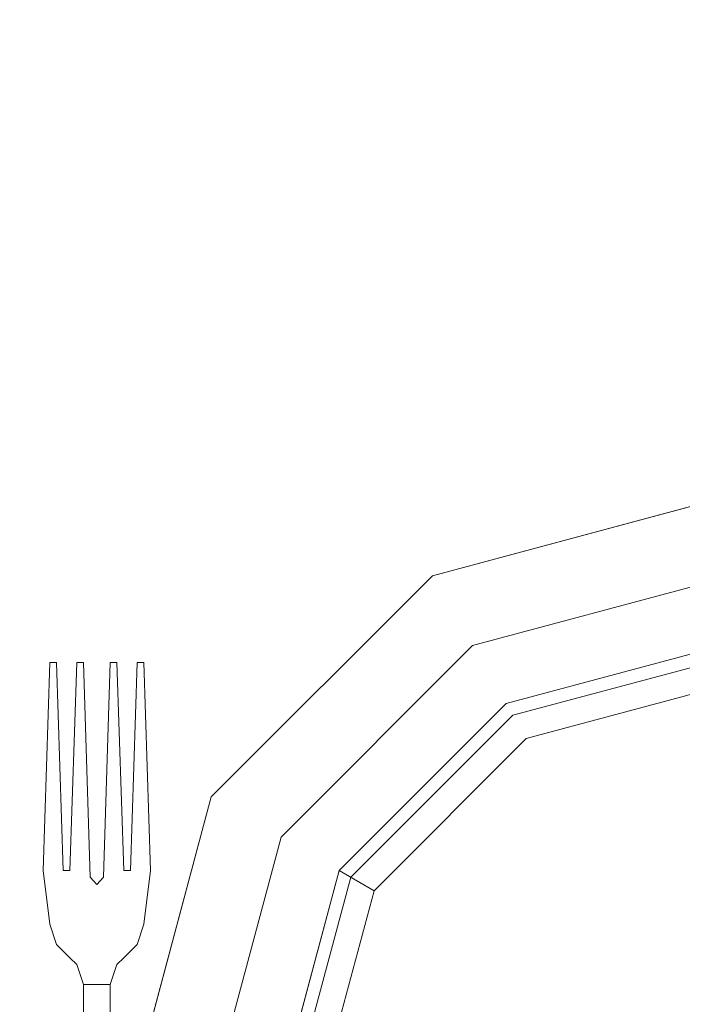
# Model space of a CAD drawing. Units: inches. Extents: x 375 to 1122, y 27 to 1069.
# Tile 87 of 155: x 719.125 to 725.203, y 854.634 to 863.668. Entities that reach past the tile are written whole.
import ezdxf

# ---------------------------------------------------------------- set-up
doc = ezdxf.new("R2010")
doc.units = ezdxf.units.IN
doc.layers.add('A-ANNO-DIMS', color=2, linetype='Continuous', lineweight=18)
doc.layers.add('Furniture', color=30, linetype='Continuous', lineweight=18)
doc.styles.get("Standard").update_dxf_attribs({"font": 'arial.ttf'})
doc.dimstyles.new('ISO-25', dxfattribs={"dimtxt": 12, "dimasz": 2.5, "dimexe": 1.5, "dimexo": 1.5, "dimtad": 1, "dimdec": 1, "dimlunit": 3, "dimtxsty": 'Standard', "dimblk": 'ARCHTICK', "dimcen": 2.5, "dimadec": 0, "dimazin": 0, "dimtfac": 1, "dimtdec": 1, "dimtmove": 0, "dimatfit": 3, "dimfxl": 1.5, "dimfxlon": 1, "dimarcsym": 0})

# ---------------------------------------------------------------- blocks, each defined once
blk = doc.blocks.new('A$C403C54AD')
for p, q in [((2.0741, 0.86135, -0.05014), (2.07871, 0.86289, -0.04968)), ((2.0741, 0.86135, -0.05322), (2.07871, 0.86289, -0.05276))]:
    blk.add_line(p, q)
at = {"linetype": 'ByBlock'}
for points, invisible_edges in [([(1.97559, 1.01834, -0.03783), (1.99406, 1.01834, -0.03783), (2.01014, 0.95832, -0.03783), (1.99415, 0.94908, -0.03783)], 5), ([(2.00945, 1.01834, -0.05168), (1.97559, 1.01834, -0.04244), (1.99415, 0.94908, -0.04244), (2.02347, 0.96601, -0.05168)], 5), ([(1.99406, 1.01834, -0.03783), (2.01253, 1.01834, -0.04398), (2.02614, 0.96755, -0.04398), (2.01014, 0.95832, -0.03783)], 5), ([(2.01868, 1.01834, -0.06091), (2.00945, 1.01834, -0.05168), (2.02347, 0.96601, -0.05168), (2.03147, 0.97063, -0.06091)], 5), ([(2.01253, 1.01834, -0.04398), (2.11411, 1.01834, -0.04398), (2.11411, 1.01834, -0.04398), (2.02614, 0.96755, -0.04398)], 5), ([(2.02614, 0.96755, -0.04398), (2.11411, 1.01834, -0.04398), (2.11411, 1.01834, -0.04398), (2.06332, 0.93037, -0.04398)], 5), ([(2.06332, 0.93037, -0.04398), (2.11411, 1.01834, -0.04398), (2.11411, 1.01834, -0.04398), (2.11411, 0.91676, -0.04398)], 5), ([(2.03147, 0.97063, -0.06091), (2.02347, 0.96601, -0.05168), (2.06178, 0.9277, -0.05168), (2.0664, 0.9357, -0.06091)], 1), ([(2.01014, 0.95832, -0.03783), (2.02614, 0.96755, -0.04398), (2.06332, 0.93037, -0.04398), (2.05409, 0.91437, -0.03783)], 5), ([(2.02347, 0.96601, -0.05168), (1.99415, 0.94908, -0.04244), (2.04485, 0.89838, -0.04244), (2.06178, 0.9277, -0.05168)], 5), ([(1.99415, 0.94908, -0.03783), (2.01014, 0.95832, -0.03783), (2.05409, 0.91437, -0.03783), (2.04485, 0.89838, -0.03783)], 5), ([(2.05409, 0.91437, -0.03783), (2.06332, 0.93037, -0.04398), (2.11411, 0.91676, -0.04398), (2.11411, 0.89829, -0.03783)], 5), ([(2.06178, 0.9277, -0.05168), (2.04485, 0.89838, -0.04244), (2.11411, 0.87982, -0.04244), (2.11411, 0.91368, -0.05168)], 5), ([(2.04485, 0.89838, -0.03783), (2.05409, 0.91437, -0.03783), (2.11411, 0.89829, -0.03783), (2.11411, 0.87982, -0.03783)], 5)]:
    blk.add_3dface(points, dxfattribs=dict(at, invisible_edges=invisible_edges))
for points in [[(1.97559, 1.01834, -0.04244), (1.97559, 1.01834, -0.03783), (1.99415, 0.94908, -0.03783), (1.99415, 0.94908, -0.04244)], [(1.99415, 0.94908, -0.04244), (1.99415, 0.94908, -0.03783), (2.04485, 0.89838, -0.03783), (2.04485, 0.89838, -0.04244)], [(2.0664, 0.9357, -0.06091), (2.06178, 0.9277, -0.05168), (2.11411, 0.91368, -0.05168), (2.11411, 0.92291, -0.06091)], [(2.04485, 0.89838, -0.04244), (2.04485, 0.89838, -0.03783), (2.11411, 0.87982, -0.03783), (2.11411, 0.87982, -0.04244)]]:
    blk.add_3dface(points, dxfattribs=at)
for points, invisible_edges in [([(2.06178, 0.87982, -0.04954), (2.06178, 0.88444, -0.04954), (2.01407, 0.8829, -0.04244), (2.01407, 0.88136, -0.04244)], 1), ([(2.06178, 0.87982, -0.05262), (2.06178, 0.88444, -0.05262), (2.01407, 0.8829, -0.04552), (2.01407, 0.88136, -0.04552)], 1), ([(2.0741, 0.8829, -0.05014), (2.06178, 0.87828, -0.04954), (2.06178, 0.87982, -0.04954), (2.06178, 0.88444, -0.04954)], 5), ([(2.0741, 0.8829, -0.05322), (2.06178, 0.87828, -0.05262), (2.06178, 0.87982, -0.05262), (2.06178, 0.88444, -0.05262)], 5), ([(2.0741, 0.8829, -0.05014), (2.0741, 0.8829, -0.05322), (2.06178, 0.88444, -0.05262), (2.06178, 0.88444, -0.04954)], 1), ([(2.0741, 0.8829, -0.05014), (2.06498, 0.87212, -0.04994), (2.06332, 0.87366, -0.04979), (2.06178, 0.87828, -0.04954)], 13), ([(2.0741, 0.8829, -0.05322), (2.06498, 0.87212, -0.05301), (2.06332, 0.87366, -0.05286), (2.06178, 0.87828, -0.05262)], 13), ([(2.0741, 0.8829, -0.05014), (2.06498, 0.87212, -0.04994), (2.0741, 0.86135, -0.05014), (2.0741, 0.8829, -0.05014)], 7), ([(2.0741, 0.8829, -0.05322), (2.06498, 0.87212, -0.05301), (2.0741, 0.86135, -0.05322), (2.0741, 0.8829, -0.05322)], 7), ([(2.07871, 0.88136, -0.04968), (2.07871, 0.86289, -0.04968), (2.0741, 0.86135, -0.05014), (2.0741, 0.8829, -0.05014)], 5), ([(2.07871, 0.88136, -0.05276), (2.07871, 0.86289, -0.05276), (2.0741, 0.86135, -0.05322), (2.0741, 0.8829, -0.05322)], 5), ([(2.07871, 0.88136, -0.05276), (2.07871, 0.88136, -0.04968), (2.0741, 0.8829, -0.05014), (2.0741, 0.8829, -0.05322)], 4), ([(2.08179, 0.86596, -0.05152), (2.08179, 0.87828, -0.05152), (2.07871, 0.88136, -0.05276), (2.07871, 0.86289, -0.05276)], 5), ([(2.08179, 0.86596, -0.04844), (2.08179, 0.87828, -0.04844), (2.07871, 0.88136, -0.04968), (2.07871, 0.86289, -0.04968)], 5), ([(2.06178, 0.87828, -0.04954), (2.06332, 0.87366, -0.04979), (2.01407, 0.8752, -0.04244), (2.01407, 0.87674, -0.04244)], 1), ([(2.06178, 0.87828, -0.05262), (2.06332, 0.87366, -0.05286), (2.01407, 0.8752, -0.04552), (2.01407, 0.87674, -0.04552)], 1), ([(2.08333, 0.8675, -0.04739), (2.08333, 0.87674, -0.04739), (2.08179, 0.87828, -0.04844), (2.08179, 0.86596, -0.04844)], 5), ([(2.08333, 0.8675, -0.05018), (2.08333, 0.87674, -0.05018), (2.08179, 0.87828, -0.05152), (2.08179, 0.86596, -0.05152)], 5), ([(2.08333, 0.87674, -0.05018), (2.08333, 0.87674, -0.04739), (2.08179, 0.87828, -0.04844), (2.08179, 0.87828, -0.05152)], 1), ([(2.08795, 0.8752, -0.04504), (2.08795, 0.86904, -0.04504), (2.08333, 0.8675, -0.04739), (2.08333, 0.87674, -0.04739)], 4), ([(2.08795, 0.8752, -0.04504), (2.08795, 0.8752, -0.04763), (2.08333, 0.87674, -0.05018), (2.08333, 0.87674, -0.04739)], 5), ([(2.08795, 0.8752, -0.04763), (2.08795, 0.86904, -0.04763), (2.08333, 0.8675, -0.05018), (2.08333, 0.87674, -0.05018)], 4), ([(2.09872, 0.8752, -0.04555), (2.09872, 0.8752, -0.04296), (2.08795, 0.8752, -0.04504), (2.08795, 0.8752, -0.04763)], 5), ([(2.0741, 0.86135, -0.05014), (2.06498, 0.87212, -0.04994), (2.06332, 0.87058, -0.04979), (2.06178, 0.86596, -0.04954)], 13), ([(2.0741, 0.86135, -0.05322), (2.06498, 0.87212, -0.05301), (2.06332, 0.87058, -0.05286), (2.06178, 0.86596, -0.05262)], 13), ([(2.06332, 0.87058, -0.04979), (2.06178, 0.86596, -0.04954), (2.01407, 0.8675, -0.04244), (2.01407, 0.86904, -0.04244)], 1), ([(2.06332, 0.87058, -0.05286), (2.06178, 0.86596, -0.05262), (2.01407, 0.8675, -0.04552), (2.01407, 0.86904, -0.04552)], 1), ([(2.08333, 0.8675, -0.04739), (2.08333, 0.8675, -0.05018), (2.08179, 0.86596, -0.05152), (2.08179, 0.86596, -0.04844)], 1), ([(2.08795, 0.86904, -0.04763), (2.08795, 0.86904, -0.04504), (2.08333, 0.8675, -0.04739), (2.08333, 0.8675, -0.05018)], 5), ([(2.08795, 0.86904, -0.04763), (2.08795, 0.86904, -0.04504), (2.09872, 0.86904, -0.04296), (2.09872, 0.86904, -0.04555)], 5), ([(2.0741, 0.86135, -0.05014), (2.06178, 0.86596, -0.04954), (2.06178, 0.86443, -0.04954), (2.06178, 0.85981, -0.04954)], 5), ([(2.0741, 0.86135, -0.05322), (2.06178, 0.86596, -0.05262), (2.06178, 0.86443, -0.05262), (2.06178, 0.85981, -0.05262)], 5), ([(2.06178, 0.86443, -0.04954), (2.06178, 0.85981, -0.04954), (2.01407, 0.86135, -0.04244), (2.01407, 0.86289, -0.04244)], 1), ([(2.06178, 0.86443, -0.05262), (2.06178, 0.85981, -0.05262), (2.01407, 0.86135, -0.04552), (2.01407, 0.86289, -0.04552)], 1), ([(2.07871, 0.86289, -0.04968), (2.07871, 0.86289, -0.05276), (2.0741, 0.86135, -0.05322), (2.0741, 0.86135, -0.05014)], 4), ([(2.0741, 0.86135, -0.05322), (2.0741, 0.86135, -0.05014), (2.06178, 0.85981, -0.04954), (2.06178, 0.85981, -0.05262)], 1)]:
    blk.add_3dface(points, dxfattribs=dict(invisible_edges=invisible_edges))
for points in [[(2.06178, 0.88444, -0.05262), (2.06178, 0.88444, -0.04954), (2.01407, 0.8829, -0.04244), (2.01407, 0.8829, -0.04552)], [(2.01407, 0.8829, -0.04552), (2.01407, 0.8829, -0.04244), (2.01407, 0.88136, -0.04244), (2.01407, 0.88136, -0.04552)], [(2.01407, 0.88136, -0.04244), (2.01407, 0.88136, -0.04552), (2.06178, 0.87982, -0.05262), (2.06178, 0.87982, -0.04954)], [(2.08179, 0.87828, -0.04844), (2.08179, 0.87828, -0.05152), (2.07871, 0.88136, -0.05276), (2.07871, 0.88136, -0.04968)], [(2.06178, 0.87828, -0.05262), (2.06178, 0.87828, -0.04954), (2.06178, 0.87982, -0.04954), (2.06178, 0.87982, -0.05262)], [(2.06178, 0.87828, -0.05262), (2.06178, 0.87828, -0.04954), (2.01407, 0.87674, -0.04244), (2.01407, 0.87674, -0.04552)], [(2.01407, 0.87674, -0.04552), (2.01407, 0.87674, -0.04244), (2.01407, 0.8752, -0.04244), (2.01407, 0.8752, -0.04552)], [(2.01407, 0.8752, -0.04552), (2.01407, 0.8752, -0.04244), (2.06332, 0.87366, -0.04979), (2.06332, 0.87366, -0.05286)], [(2.09872, 0.86904, -0.04296), (2.09872, 0.8752, -0.04296), (2.08795, 0.8752, -0.04504), (2.08795, 0.86904, -0.04504)], [(2.09872, 0.86904, -0.04555), (2.09872, 0.8752, -0.04555), (2.08795, 0.8752, -0.04763), (2.08795, 0.86904, -0.04763)], [(2.06498, 0.87212, -0.05301), (2.06498, 0.87212, -0.04994), (2.06332, 0.87366, -0.04979), (2.06332, 0.87366, -0.05286)], [(2.06332, 0.87058, -0.04979), (2.06332, 0.87058, -0.05286), (2.06498, 0.87212, -0.05301), (2.06498, 0.87212, -0.04994)], [(2.06332, 0.87058, -0.05286), (2.06332, 0.87058, -0.04979), (2.01407, 0.86904, -0.04244), (2.01407, 0.86904, -0.04552)], [(2.01407, 0.86904, -0.04552), (2.01407, 0.86904, -0.04244), (2.01407, 0.8675, -0.04244), (2.01407, 0.8675, -0.04552)], [(2.01407, 0.8675, -0.04244), (2.01407, 0.8675, -0.04552), (2.06178, 0.86596, -0.05262), (2.06178, 0.86596, -0.04954)], [(2.06178, 0.86443, -0.04954), (2.06178, 0.86443, -0.05262), (2.06178, 0.86596, -0.05262), (2.06178, 0.86596, -0.04954)], [(2.08179, 0.86596, -0.05152), (2.08179, 0.86596, -0.04844), (2.07871, 0.86289, -0.04968), (2.07871, 0.86289, -0.05276)], [(2.06178, 0.86443, -0.04954), (2.06178, 0.86443, -0.05262), (2.01407, 0.86289, -0.04552), (2.01407, 0.86289, -0.04244)], [(2.01407, 0.86289, -0.04552), (2.01407, 0.86289, -0.04244), (2.01407, 0.86135, -0.04244), (2.01407, 0.86135, -0.04552)], [(2.01407, 0.86135, -0.04244), (2.01407, 0.86135, -0.04552), (2.06178, 0.85981, -0.05262), (2.06178, 0.85981, -0.04954)]]:
    blk.add_3dface(points)
blk = doc.blocks.new('_ArchTick')
at = {"color": 0, "linetype": 'ByBlock', "const_width": 0.15}
blk.add_lwpolyline([(-0.5, -0.5), (0.5, 0.5)], dxfattribs=at)
blk = doc.blocks.new('*D85')
at = {"layer": 'A-ANNO-DIMS', "color": 0, "lineweight": -2, "transparency": 16777216}
for p, q in [((401.5073, 868.5277), (398.5073, 868.5277)), ((400.0073, 814.5277), (400.0073, 868.5277)), ((401.5073, 814.5277), (398.5073, 814.5277))]:
    blk.add_line(p, q, dxfattribs=at)
at = {"layer": 'Defpoints', "color": 0, "transparency": 16777216}
for p in [(400.0073, 868.5277), (845.0073, 868.5277), (845.0073, 814.5277)]:
    blk.add_point(p, dxfattribs=at)
at = {"layer": 'A-ANNO-DIMS', "color": 0, "lineweight": -2, "transparency": 16777216, "xscale": 2.5, "yscale": 2.5, "zscale": 2.5}
for p, rotation in [((400.0073, 868.5277), 90), ((400.0073, 814.5277), 270)]:
    blk.add_blockref('_ArchTick', p, dxfattribs=dict(at, rotation=rotation))
at = {"layer": 'A-ANNO-DIMS', "color": 0, "transparency": 16777216, "insert": (393.2555, 841.5277), "char_height": 12, "attachment_point": 5, "rotation": 90}
blk.add_mtext('4\'-6"', dxfattribs=at)

msp = doc.modelspace()

# ---------------------------------------------------------------- block references
at = {"layer": 'Furniture', "xscale": 39.9918517141215, "yscale": 39.9918517141215, "zscale": 39.9918517141215, "rotation": 270}
msp.add_blockref('A$C403C54AD', (684.9549, 938.3156, 0.024), dxfattribs=at)

# ---------------------------------------------------------------- dimensions: what is measured, and where the dimension line sits
at = {"layer": 'A-ANNO-DIMS'}
dim = msp.add_linear_dim(base=(400.0073, 868.5277), p1=(845.0073, 814.5277), p2=(845.0073, 868.5277), angle=90, dimstyle='ISO-25', override={"dimdec": 1, "dimlfac": 1, "dimrnd": 0, "dimzin": 1, "dimdsep": 46, "dimlunit": 4, "dimfrac": 2}, dxfattribs=at)
dim.commit()
dim.dimension.update_dxf_attribs({"geometry": '*D85', "text_midpoint": (393.2555, 841.5277)})

doc.saveas('drawing.dxf')
